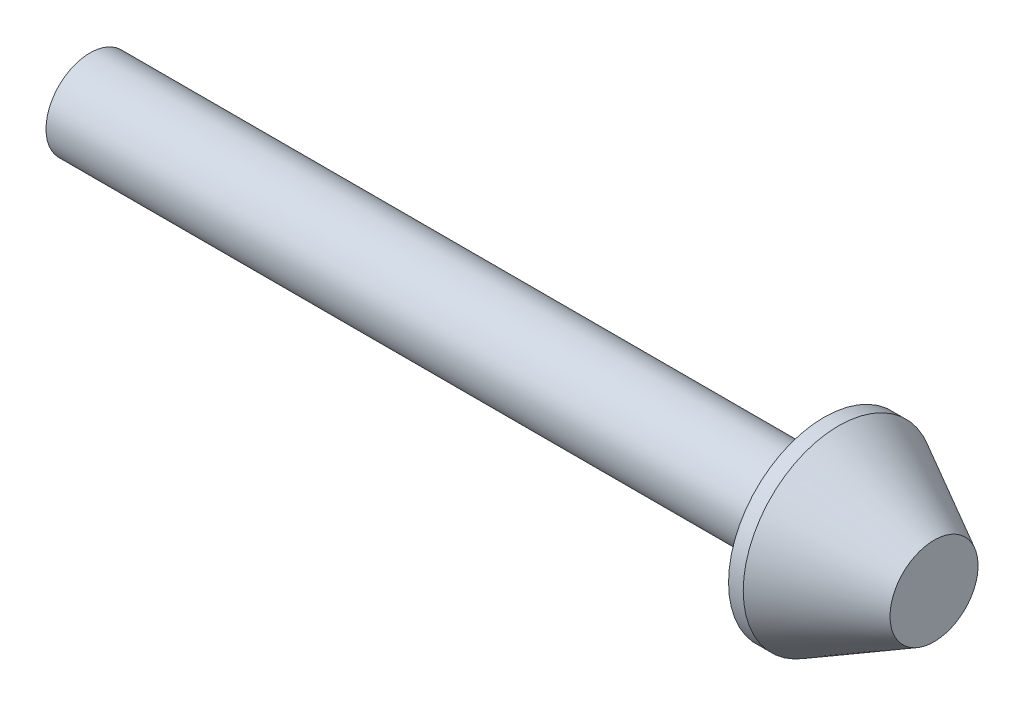
from build123d import *


with BuildPart() as part:
    # Rod Profile Sketch → Rod Body Revolve (revolve)
    with BuildSketch(Plane.XY, mode=Mode.PRIVATE) as rod_body_revolve_sk:
        Polygon((0, 0), (115, 0), (115, 6), (102, 13), (100, 13), (100, 6), (0, 6), align=None)
    revolve(rod_body_revolve_sk.sketch.rotate(Axis((0, 0, 0), (1, 0, 0)), 90), axis=Axis((0, 0, 0), (1, 0, 0)))


solid = part.part
